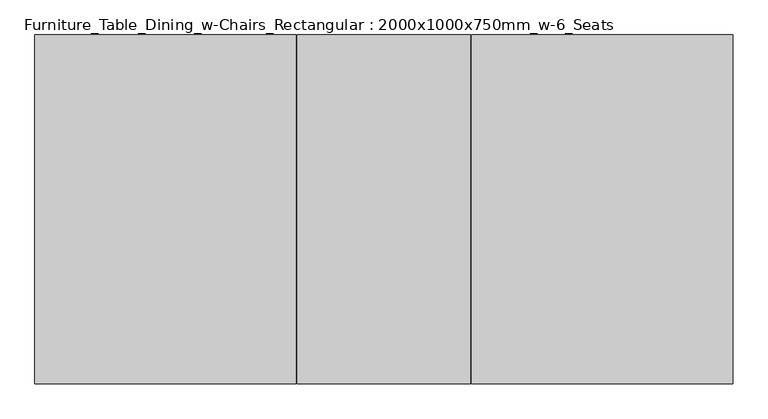
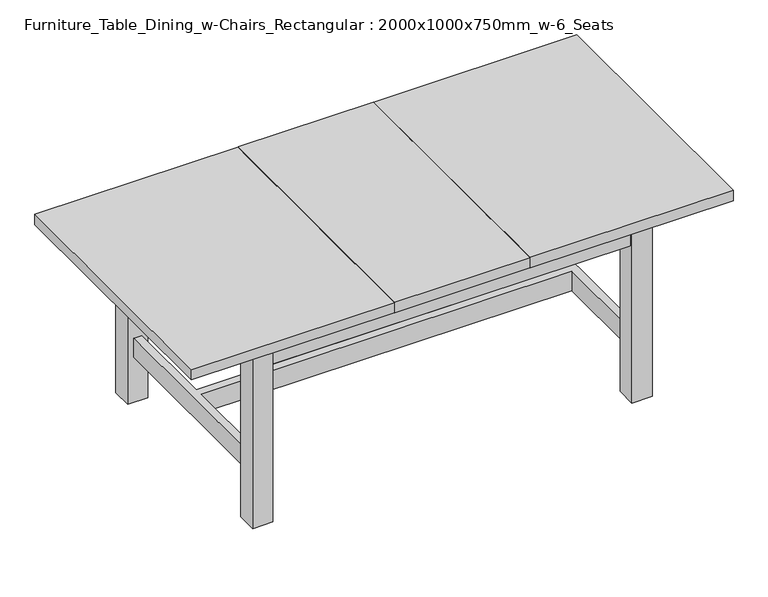
"""IFC4 building model written with IfcOpenShell, lengths in millimetres: furniture geometry, Furniture_Table_Dining_w-Chairs_Rectangular : 2000x1000x750mm_w-6_Seats."""

from ifc_helpers import new_model, si_unit, frame, origin, origin_with_axes, place, context, project, spatial, polyline, outline, extrude, faceted_brep, source, transform, mapped, element, save


def furniture_table_dining_w_chairs_rectangular_2000x1000x750mm_b8cbee69(model_context):
    return source(origin(), model_context, "Body", "SolidModel", [
        faceted_brep([(1118.1787219, -455.6453708, 750.0), (1118.1787219, 544.3546292, 750.0), (369.6787219, 544.3546292, 750.0), (369.6787219, -455.6453708, 750.0), (-881.8212781, 544.3546292, 750.0), (-881.8212781, -455.6453708, 750.0), (-133.3212781, -455.6453708, 750.0), (-133.3212781, 544.3546292, 750.0), (366.6787219, 544.3546292, 750.0), (-130.3212781, 544.3546292, 750.0), (-130.3212781, -455.6453708, 750.0), (366.6787219, -455.6453708, 750.0), (-881.8212781, -455.6453708, 710.0), (-881.8212781, 544.3546292, 710.0), (-133.3212781, 544.3546292, 710.0), (-131.8212781, 542.8546292, 710.0), (-130.3212781, 544.3546292, 710.0), (366.6787219, 544.3546292, 710.0), (368.1787219, 542.8546292, 710.0), (369.6787219, 544.3546292, 710.0), (1118.1787219, 544.3546292, 710.0), (1118.1787219, -455.6453708, 710.0), (369.6787219, -455.6453708, 710.0), (368.1787219, -454.1453708, 710.0), (366.6787219, -455.6453708, 710.0), (-130.3212781, -455.6453708, 710.0), (-131.8212781, -454.1453708, 710.0), (-133.3212781, -455.6453708, 710.0), (-131.8212781, 542.8546292, 748.5), (368.1787219, 542.8546292, 748.5), (-131.8212781, -454.1453708, 748.5), (368.1787219, -454.1453708, 748.5)], [[[0, 1, 2, 3]], [[4, 5, 6, 7]], [[8, 9, 10, 11]], [[12, 13, 14, 15, 16, 17, 18, 19, 20, 21, 22, 23, 24, 25, 26, 27]], [[1, 0, 21, 20]], [[9, 8, 17, 16]], [[1, 20, 19, 2]], [[13, 4, 7, 14]], [[5, 4, 13, 12]], [[11, 10, 25, 24]], [[21, 0, 3, 22]], [[5, 12, 27, 6]], [[15, 28, 9, 16]], [[28, 15, 14, 7]], [[18, 29, 2, 19]], [[29, 18, 17, 8]], [[9, 28, 30, 10]], [[28, 7, 6, 30]], [[2, 29, 31, 3]], [[29, 8, 11, 31]], [[10, 30, 26, 25]], [[30, 6, 27, 26]], [[3, 31, 23, 22]], [[31, 11, 24, 23]]]),
        extrude(outline(polyline([(-544.3212781, -393.1453708), (-619.3212781, -393.1453708), (-619.3212781, -318.1453708), (-544.3212781, -318.1453708), (-544.3212781, -393.1453708)])), origin_with_axes(), (0.0, 0.0, 1.0), 710.0),
        extrude(outline(polyline([(780.6787219, 481.8546292), (855.6787219, 481.8546292), (855.6787219, 406.8546292), (780.6787219, 406.8546292), (780.6787219, 481.8546292)])), origin_with_axes(), (0.0, 0.0, 1.0), 710.0),
        extrude(outline(polyline([(780.6787219, -318.1453708), (855.6787219, -318.1453708), (855.6787219, -393.1453708), (780.6787219, -393.1453708), (780.6787219, -318.1453708)])), origin_with_axes(), (0.0, 0.0, 1.0), 710.0),
        extrude(outline(polyline([(-544.3212781, 481.8546292), (-544.3212781, 406.8546292), (-619.3212781, 406.8546292), (-619.3212781, 481.8546292), (-544.3212781, 481.8546292)])), origin_with_axes(), (0.0, 0.0, 1.0), 710.0),
        extrude(outline(polyline([(-566.8212781, -318.1453708), (-596.8212781, -318.1453708), (-596.8212781, 406.8546292), (-566.8212781, 406.8546292), (-566.8212781, 59.3546292), (803.1787219, 59.3546292), (803.1787219, 406.8546292), (833.1787219, 406.8546292), (833.1787219, -318.1453708), (803.1787219, -318.1453708), (803.1787219, 29.3546292), (-566.8212781, 29.3546292), (-566.8212781, -318.1453708)])), frame((0.0, 0.0, 175.0), z_axis=(0.0, 0.0, 1.0), x_axis=(1.0, 0.0, 0.0)), (0.0, 0.0, 1.0), 75.0),
        extrude(outline(polyline([(-544.3212781, 474.3546292), (780.6787219, 474.3546292), (780.6787219, 454.3546292), (-544.3212781, 454.3546292), (-544.3212781, 474.3546292)])), frame((0.0, 0.0, 610.0), z_axis=(0.0, 0.0, 1.0), x_axis=(1.0, 0.0, 0.0)), (0.0, 0.0, 1.0), 100.0),
        extrude(outline(polyline([(-611.8212781, -318.1453708), (-611.8212781, 406.8546292), (-591.8212781, 406.8546292), (-591.8212781, -318.1453708), (-611.8212781, -318.1453708)])), frame((0.0, 0.0, 610.0), z_axis=(0.0, 0.0, 1.0), x_axis=(1.0, 0.0, 0.0)), (0.0, 0.0, 1.0), 100.0),
        extrude(outline(polyline([(780.6787219, -385.6453708), (-544.3212781, -385.6453708), (-544.3212781, -365.6453708), (780.6787219, -365.6453708), (780.6787219, -385.6453708)])), frame((0.0, 0.0, 610.0), z_axis=(0.0, 0.0, 1.0), x_axis=(1.0, 0.0, 0.0)), (0.0, 0.0, 1.0), 100.0),
        extrude(outline(polyline([(848.1787219, 406.8546292), (848.1787219, -318.1453708), (828.1787219, -318.1453708), (828.1787219, 406.8546292), (848.1787219, 406.8546292)])), frame((0.0, 0.0, 610.0), z_axis=(0.0, 0.0, 1.0), x_axis=(1.0, 0.0, 0.0)), (0.0, 0.0, 1.0), 100.0),
    ])


if __name__ == "__main__":
    model = new_model("IFC4")
    model_context = context("Model", 3, world=origin())
    ifc_project = project(units=[si_unit("LENGTHUNIT", "METRE", prefix="MILLI")], contexts=[model_context])
    site = spatial("IfcSite", under=ifc_project)
    building = spatial("IfcBuilding", under=site)
    placement = place(None, origin())
    furniture_table_dining_w_chairs_rectangular_2000x1000x750mm_shape = furniture_table_dining_w_chairs_rectangular_2000x1000x750mm_b8cbee69(model_context)
    element("IfcFurniture", 1, ObjectType="Furniture_Table_Dining_w-Chairs_Rectangular : 2000x1000x750mm_w-6_Seats", at=placement, inside=building, context=model_context, shape_type="MappedRepresentation", body=[
        mapped(furniture_table_dining_w_chairs_rectangular_2000x1000x750mm_shape, transform((0.0, 0.0, 0.0), x_axis=(1.0, 0.0, 0.0), y_axis=(0.0, 1.0, 0.0), z_axis=(0.0, 0.0, 1.0))),
    ])
    save(model, "model.ifc")

# Revit data of these elements
# Type "Furniture_Table_Dining_w-Chairs_Rectangular : 2000x1000x750mm_w-6_Seats"
#   Keynote = "N"
#   Width = 1000 mm
#   Table Top Thickness = 40 mm
#   Table Height = 750 mm
#   Length = 2000 mm
#   Leg Width = 75 mm
#   Leg Spacing Width = 800 mm
#   Leg Spacing Length = 1400 mm
#   Chair Side Spacing = 700 mm
#   Centre Piece = 500 mm
#   Vis - End Chairs = yes
#   Material Table = Wood - Birch
#   Material Chair Structure = Wood - Birch
#   Material Chair Covering = Fabric - Beige
#   Default Elevation = 0
# Element 1 (IfcFurniture, "Furniture_Table_Dining_w-Chairs_Rectangular : 2000x1000x750mm_w-6_Seats")
#   Materials on its faces: "Wood - Birch"
# Materials
#   "Wood - Birch": colour RGB 210 159 95, transparency 0
#   "Fabric - Beige": class "Fabric", colour RGB 231 227 195, transparency 0
